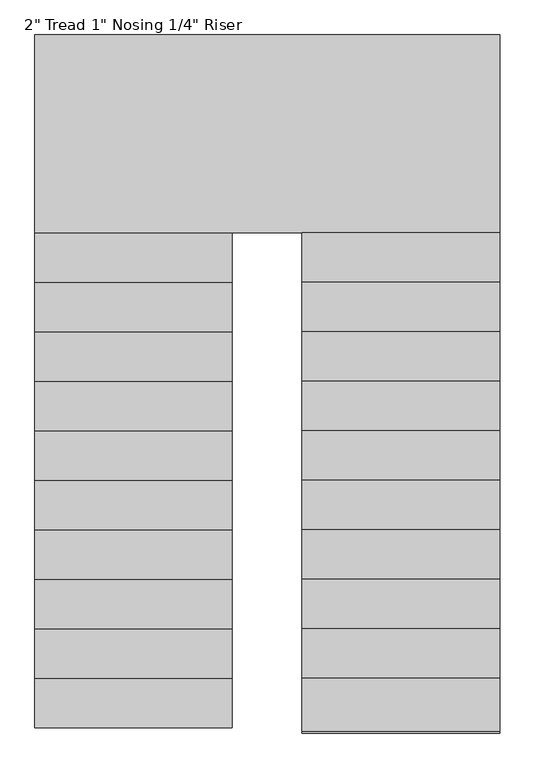
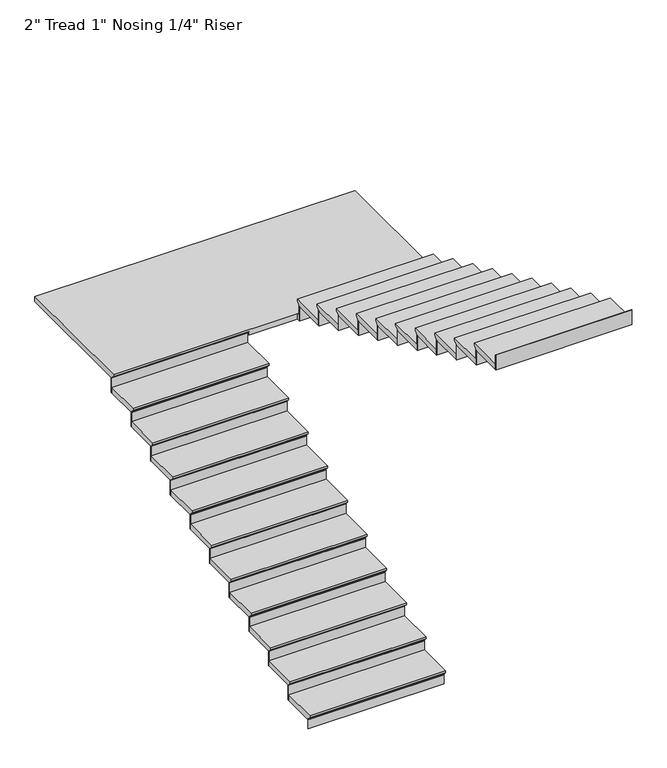
"""IFC4 building model written with IfcOpenShell, lengths in millimetres: stair flight geometry."""

from ifc_helpers import new_model, si_unit, origin, place, context, project, spatial, faceted_brep, source, transform, mapped, element, save


def stair_flight_b17f4745(model_context):
    return source(origin(), model_context, "Body", "Brep", [
        faceted_brep([(-629.5987998, 3364.6067329, 9720.6954545), (-629.5987998, 3364.6067329, 9739.7454545), (-1845.5417538, 3364.6067329, 9739.7454545), (-1845.5417538, 3364.6067329, 9720.6954545), (-629.5987998, 3390.0067329, 9695.2954545), (-1845.5417538, 3390.0067329, 9695.2954545), (-629.5987998, 3694.8067329, 9739.7454545), (-1845.5417538, 3694.8067329, 9739.7454545), (-1845.5417538, 3390.0067329, 9688.9454545), (-1845.5417538, 3694.8067329, 9688.9454545), (-629.5987998, 3694.8067329, 9688.9454545), (-629.5987998, 3390.0067329, 9688.9454545)], [[[0, 1, 2, 3]], [[4, 0, 3, 5]], [[2, 1, 6, 7]], [[8, 9, 10, 11]], [[2, 7, 9, 8, 5, 3]], [[8, 11, 4, 5]], [[6, 1, 0, 4, 11, 10]], [[7, 6, 10, 9]]]),
        faceted_brep([(-629.5987998, 3390.0067329, 9688.9454545), (-629.5987998, 3390.0067329, 9601.2), (-629.5987998, 3396.3567329, 9601.2), (-629.5987998, 3396.3567329, 9688.9454545), (-1845.5417538, 3390.0067329, 9688.9454545), (-1845.5417538, 3396.3567329, 9688.9454545), (-1845.5417538, 3396.3567329, 9601.2), (-1845.5417538, 3390.0067329, 9601.2)], [[[0, 1, 2, 3]], [[4, 5, 6, 7]], [[1, 0, 4, 7]], [[2, 1, 7, 6]], [[3, 2, 6, 5]], [[0, 3, 5, 4]]]),
        faceted_brep([(-629.5987998, 3694.8067329, 9827.4909091), (-629.5987998, 3694.8067329, 9688.9454545), (-629.5987998, 3701.1567329, 9688.9454545), (-629.5987998, 3701.1567329, 9827.4909091), (-1845.5417538, 3694.8067329, 9827.4909091), (-1845.5417538, 3701.1567329, 9827.4909091), (-1845.5417538, 3701.1567329, 9688.9454545), (-1845.5417538, 3694.8067329, 9688.9454545)], [[[0, 1, 2, 3]], [[4, 5, 6, 7]], [[1, 0, 4, 7]], [[2, 1, 7, 6]], [[3, 2, 6, 5]], [[0, 3, 5, 4]]]),
        faceted_brep([(-1845.5417538, 3669.4067329, 9878.2909091), (-629.5987998, 3669.4067329, 9878.2909091), (-629.5987998, 3999.6067329, 9878.2909091), (-1845.5417538, 3999.6067329, 9878.2909091), (-1845.5417538, 3694.8067329, 9827.4909091), (-1845.5417538, 3999.6067329, 9827.4909091), (-629.5987998, 3999.6067329, 9827.4909091), (-629.5987998, 3694.8067329, 9827.4909091), (-1845.5417538, 3694.8067329, 9833.8409091), (-1845.5417538, 3669.4067329, 9859.2409091), (-629.5987998, 3694.8067329, 9833.8409091), (-629.5987998, 3669.4067329, 9859.2409091)], [[[0, 1, 2, 3]], [[4, 5, 6, 7]], [[0, 3, 5, 4, 8, 9]], [[4, 7, 10, 8]], [[2, 1, 11, 10, 7, 6]], [[3, 2, 6, 5]], [[11, 1, 0, 9]], [[10, 11, 9, 8]]]),
        faceted_brep([(-629.5987998, 3999.6067329, 9966.0363636), (-629.5987998, 3999.6067329, 9827.4909091), (-629.5987998, 4005.9567329, 9827.4909091), (-629.5987998, 4005.9567329, 9966.0363636), (-1845.5417538, 3999.6067329, 9966.0363636), (-1845.5417538, 4005.9567329, 9966.0363636), (-1845.5417538, 4005.9567329, 9827.4909091), (-1845.5417538, 3999.6067329, 9827.4909091)], [[[0, 1, 2, 3]], [[4, 5, 6, 7]], [[1, 0, 4, 7]], [[2, 1, 7, 6]], [[3, 2, 6, 5]], [[0, 3, 5, 4]]]),
        faceted_brep([(-1845.5417538, 3974.2067329, 10016.8363636), (-629.5987998, 3974.2067329, 10016.8363636), (-629.5987998, 4304.4067329, 10016.8363636), (-1845.5417538, 4304.4067329, 10016.8363636), (-1845.5417538, 3999.6067329, 9966.0363636), (-1845.5417538, 4304.4067329, 9966.0363636), (-629.5987998, 4304.4067329, 9966.0363636), (-629.5987998, 3999.6067329, 9966.0363636), (-1845.5417538, 3999.6067329, 9972.3863636), (-1845.5417538, 3974.2067329, 9997.7863636), (-629.5987998, 3999.6067329, 9972.3863636), (-629.5987998, 3974.2067329, 9997.7863636)], [[[0, 1, 2, 3]], [[4, 5, 6, 7]], [[0, 3, 5, 4, 8, 9]], [[4, 7, 10, 8]], [[2, 1, 11, 10, 7, 6]], [[3, 2, 6, 5]], [[11, 1, 0, 9]], [[10, 11, 9, 8]]]),
        faceted_brep([(-629.5987998, 4304.4067329, 10104.5818182), (-629.5987998, 4304.4067329, 9966.0363636), (-629.5987998, 4310.7567329, 9966.0363636), (-629.5987998, 4310.7567329, 10104.5818182), (-1845.5417538, 4304.4067329, 10104.5818182), (-1845.5417538, 4310.7567329, 10104.5818182), (-1845.5417538, 4310.7567329, 9966.0363636), (-1845.5417538, 4304.4067329, 9966.0363636)], [[[0, 1, 2, 3]], [[4, 5, 6, 7]], [[1, 0, 4, 7]], [[2, 1, 7, 6]], [[3, 2, 6, 5]], [[0, 3, 5, 4]]]),
        faceted_brep([(-1845.5417538, 4279.0067329, 10155.3818182), (-629.5987998, 4279.0067329, 10155.3818182), (-629.5987998, 4609.2067329, 10155.3818182), (-1845.5417538, 4609.2067329, 10155.3818182), (-1845.5417538, 4304.4067329, 10104.5818182), (-1845.5417538, 4609.2067329, 10104.5818182), (-629.5987998, 4609.2067329, 10104.5818182), (-629.5987998, 4304.4067329, 10104.5818182), (-1845.5417538, 4304.4067329, 10110.9318182), (-1845.5417538, 4279.0067329, 10136.3318182), (-629.5987998, 4304.4067329, 10110.9318182), (-629.5987998, 4279.0067329, 10136.3318182)], [[[0, 1, 2, 3]], [[4, 5, 6, 7]], [[0, 3, 5, 4, 8, 9]], [[4, 7, 10, 8]], [[2, 1, 11, 10, 7, 6]], [[3, 2, 6, 5]], [[11, 1, 0, 9]], [[10, 11, 9, 8]]]),
        faceted_brep([(-629.5987998, 4609.2067329, 10243.1272727), (-629.5987998, 4609.2067329, 10104.5818182), (-629.5987998, 4615.5567329, 10104.5818182), (-629.5987998, 4615.5567329, 10243.1272727), (-1845.5417538, 4609.2067329, 10243.1272727), (-1845.5417538, 4615.5567329, 10243.1272727), (-1845.5417538, 4615.5567329, 10104.5818182), (-1845.5417538, 4609.2067329, 10104.5818182)], [[[0, 1, 2, 3]], [[4, 5, 6, 7]], [[1, 0, 4, 7]], [[2, 1, 7, 6]], [[3, 2, 6, 5]], [[0, 3, 5, 4]]]),
        faceted_brep([(-1845.5417538, 4583.8067329, 10293.9272727), (-629.5987998, 4583.8067329, 10293.9272727), (-629.5987998, 4914.0067329, 10293.9272727), (-1845.5417538, 4914.0067329, 10293.9272727), (-1845.5417538, 4609.2067329, 10243.1272727), (-1845.5417538, 4914.0067329, 10243.1272727), (-629.5987998, 4914.0067329, 10243.1272727), (-629.5987998, 4609.2067329, 10243.1272727), (-1845.5417538, 4609.2067329, 10249.4772727), (-1845.5417538, 4583.8067329, 10274.8772727), (-629.5987998, 4609.2067329, 10249.4772727), (-629.5987998, 4583.8067329, 10274.8772727)], [[[0, 1, 2, 3]], [[4, 5, 6, 7]], [[0, 3, 5, 4, 8, 9]], [[4, 7, 10, 8]], [[2, 1, 11, 10, 7, 6]], [[3, 2, 6, 5]], [[11, 1, 0, 9]], [[10, 11, 9, 8]]]),
        faceted_brep([(-629.5987998, 4914.0067329, 10381.6727273), (-629.5987998, 4914.0067329, 10243.1272727), (-629.5987998, 4920.3567329, 10243.1272727), (-629.5987998, 4920.3567329, 10381.6727273), (-1845.5417538, 4914.0067329, 10381.6727273), (-1845.5417538, 4920.3567329, 10381.6727273), (-1845.5417538, 4920.3567329, 10243.1272727), (-1845.5417538, 4914.0067329, 10243.1272727)], [[[0, 1, 2, 3]], [[4, 5, 6, 7]], [[1, 0, 4, 7]], [[2, 1, 7, 6]], [[3, 2, 6, 5]], [[0, 3, 5, 4]]]),
        faceted_brep([(-1845.5417538, 4888.6067329, 10432.4727273), (-629.5987998, 4888.6067329, 10432.4727273), (-629.5987998, 5218.8067329, 10432.4727273), (-1845.5417538, 5218.8067329, 10432.4727273), (-1845.5417538, 4914.0067329, 10381.6727273), (-1845.5417538, 5218.8067329, 10381.6727273), (-629.5987998, 5218.8067329, 10381.6727273), (-629.5987998, 4914.0067329, 10381.6727273), (-1845.5417538, 4914.0067329, 10388.0227273), (-1845.5417538, 4888.6067329, 10413.4227273), (-629.5987998, 4914.0067329, 10388.0227273), (-629.5987998, 4888.6067329, 10413.4227273)], [[[0, 1, 2, 3]], [[4, 5, 6, 7]], [[0, 3, 5, 4, 8, 9]], [[4, 7, 10, 8]], [[2, 1, 11, 10, 7, 6]], [[3, 2, 6, 5]], [[11, 1, 0, 9]], [[10, 11, 9, 8]]]),
        faceted_brep([(-629.5987998, 5218.8067329, 10520.2181818), (-629.5987998, 5218.8067329, 10381.6727273), (-629.5987998, 5225.1567329, 10381.6727273), (-629.5987998, 5225.1567329, 10520.2181818), (-1845.5417538, 5218.8067329, 10520.2181818), (-1845.5417538, 5225.1567329, 10520.2181818), (-1845.5417538, 5225.1567329, 10381.6727273), (-1845.5417538, 5218.8067329, 10381.6727273)], [[[0, 1, 2, 3]], [[4, 5, 6, 7]], [[1, 0, 4, 7]], [[2, 1, 7, 6]], [[3, 2, 6, 5]], [[0, 3, 5, 4]]]),
        faceted_brep([(-1845.5417538, 5193.4067329, 10571.0181818), (-629.5987998, 5193.4067329, 10571.0181818), (-629.5987998, 5523.6067329, 10571.0181818), (-1845.5417538, 5523.6067329, 10571.0181818), (-1845.5417538, 5218.8067329, 10520.2181818), (-1845.5417538, 5523.6067329, 10520.2181818), (-629.5987998, 5523.6067329, 10520.2181818), (-629.5987998, 5218.8067329, 10520.2181818), (-1845.5417538, 5218.8067329, 10526.5681818), (-1845.5417538, 5193.4067329, 10551.9681818), (-629.5987998, 5218.8067329, 10526.5681818), (-629.5987998, 5193.4067329, 10551.9681818)], [[[0, 1, 2, 3]], [[4, 5, 6, 7]], [[0, 3, 5, 4, 8, 9]], [[4, 7, 10, 8]], [[2, 1, 11, 10, 7, 6]], [[3, 2, 6, 5]], [[11, 1, 0, 9]], [[10, 11, 9, 8]]]),
        faceted_brep([(-629.5987998, 5523.6067329, 10658.7636364), (-629.5987998, 5523.6067329, 10520.2181818), (-629.5987998, 5529.9567329, 10520.2181818), (-629.5987998, 5529.9567329, 10658.7636364), (-1845.5417538, 5523.6067329, 10658.7636364), (-1845.5417538, 5529.9567329, 10658.7636364), (-1845.5417538, 5529.9567329, 10520.2181818), (-1845.5417538, 5523.6067329, 10520.2181818)], [[[0, 1, 2, 3]], [[4, 5, 6, 7]], [[1, 0, 4, 7]], [[2, 1, 7, 6]], [[3, 2, 6, 5]], [[0, 3, 5, 4]]]),
        faceted_brep([(-1845.5417538, 5498.2067329, 10709.5636364), (-629.5987998, 5498.2067329, 10709.5636364), (-629.5987998, 5828.4067329, 10709.5636364), (-1845.5417538, 5828.4067329, 10709.5636364), (-1845.5417538, 5523.6067329, 10658.7636364), (-1845.5417538, 5828.4067329, 10658.7636364), (-629.5987998, 5828.4067329, 10658.7636364), (-629.5987998, 5523.6067329, 10658.7636364), (-1845.5417538, 5523.6067329, 10665.1136364), (-1845.5417538, 5498.2067329, 10690.5136364), (-629.5987998, 5523.6067329, 10665.1136364), (-629.5987998, 5498.2067329, 10690.5136364)], [[[0, 1, 2, 3]], [[4, 5, 6, 7]], [[0, 3, 5, 4, 8, 9]], [[4, 7, 10, 8]], [[2, 1, 11, 10, 7, 6]], [[3, 2, 6, 5]], [[11, 1, 0, 9]], [[10, 11, 9, 8]]]),
        faceted_brep([(-629.5987998, 5828.4067329, 10797.3090909), (-629.5987998, 5828.4067329, 10658.7636364), (-629.5987998, 5834.7567329, 10658.7636364), (-629.5987998, 5834.7567329, 10797.3090909), (-1845.5417538, 5828.4067329, 10797.3090909), (-1845.5417538, 5834.7567329, 10797.3090909), (-1845.5417538, 5834.7567329, 10658.7636364), (-1845.5417538, 5828.4067329, 10658.7636364)], [[[0, 1, 2, 3]], [[4, 5, 6, 7]], [[1, 0, 4, 7]], [[2, 1, 7, 6]], [[3, 2, 6, 5]], [[0, 3, 5, 4]]]),
        faceted_brep([(-1845.5417538, 5803.0067329, 10848.1090909), (-629.5987998, 5803.0067329, 10848.1090909), (-629.5987998, 6133.2067329, 10848.1090909), (-1845.5417538, 6133.2067329, 10848.1090909), (-1845.5417538, 5828.4067329, 10797.3090909), (-1845.5417538, 6133.2067329, 10797.3090909), (-629.5987998, 6133.2067329, 10797.3090909), (-629.5987998, 5828.4067329, 10797.3090909), (-1845.5417538, 5828.4067329, 10803.6590909), (-1845.5417538, 5803.0067329, 10829.0590909), (-629.5987998, 5828.4067329, 10803.6590909), (-629.5987998, 5803.0067329, 10829.0590909)], [[[0, 1, 2, 3]], [[4, 5, 6, 7]], [[0, 3, 5, 4, 8, 9]], [[4, 7, 10, 8]], [[2, 1, 11, 10, 7, 6]], [[3, 2, 6, 5]], [[11, 1, 0, 9]], [[10, 11, 9, 8]]]),
        faceted_brep([(-629.5987998, 6133.2067329, 10935.8545455), (-629.5987998, 6133.2067329, 10797.3090909), (-629.5987998, 6139.5567329, 10797.3090909), (-629.5987998, 6139.5567329, 10935.8545455), (-1845.5417538, 6133.2067329, 10935.8545455), (-1845.5417538, 6139.5567329, 10935.8545455), (-1845.5417538, 6139.5567329, 10797.3090909), (-1845.5417538, 6133.2067329, 10797.3090909)], [[[0, 1, 2, 3]], [[4, 5, 6, 7]], [[1, 0, 4, 7]], [[2, 1, 7, 6]], [[3, 2, 6, 5]], [[0, 3, 5, 4]]]),
        faceted_brep([(-1845.5417538, 6107.8067329, 10986.6545455), (-629.5987998, 6107.8067329, 10986.6545455), (-629.5987998, 6438.0067329, 10986.6545455), (-1845.5417538, 6438.0067329, 10986.6545455), (-1845.5417538, 6133.2067329, 10935.8545455), (-1845.5417538, 6438.0067329, 10935.8545455), (-629.5987998, 6438.0067329, 10935.8545455), (-629.5987998, 6133.2067329, 10935.8545455), (-1845.5417538, 6133.2067329, 10942.2045455), (-1845.5417538, 6107.8067329, 10967.6045455), (-629.5987998, 6133.2067329, 10942.2045455), (-629.5987998, 6107.8067329, 10967.6045455)], [[[0, 1, 2, 3]], [[4, 5, 6, 7]], [[0, 3, 5, 4, 8, 9]], [[4, 7, 10, 8]], [[2, 1, 11, 10, 7, 6]], [[3, 2, 6, 5]], [[11, 1, 0, 9]], [[10, 11, 9, 8]]]),
        faceted_brep([(-629.5987998, 6438.0067329, 11074.4), (-629.5987998, 6438.0067329, 10935.8545455), (-629.5987998, 6444.3567329, 10935.8545455), (-629.5987998, 6444.3567329, 11074.4), (-1845.5417538, 6438.0067329, 11074.4), (-1845.5417538, 6444.3567329, 11074.4), (-1845.5417538, 6444.3567329, 10935.8545455), (-1845.5417538, 6438.0067329, 10935.8545455)], [[[0, 1, 2, 3]], [[4, 5, 6, 7]], [[1, 0, 4, 7]], [[2, 1, 7, 6]], [[3, 2, 6, 5]], [[0, 3, 5, 4]]]),
        faceted_brep([(1021.4012085, 6387.2067329, 11125.2), (1021.4012085, 7631.8067329, 11125.2), (-1845.5417538, 7631.8067329, 11125.2), (-1845.5417538, 6412.6067329, 11125.2), (-197.7987915, 6412.6067329, 11125.2), (-197.7987915, 6387.2067329, 11125.2), (1021.4012085, 7631.8067329, 11074.4), (1021.4012085, 6387.2067329, 11074.4), (-197.7987915, 6387.2067329, 11074.4), (-197.7987915, 6412.6067329, 11074.4), (-629.5987998, 6412.6067329, 11074.4), (-629.5987998, 6438.0067329, 11074.4), (-1845.5417538, 6438.0067329, 11074.4), (-1845.5417538, 7631.8067329, 11074.4), (-629.5987998, 6438.0067329, 11080.75), (-1845.5417538, 6438.0067329, 11080.75), (-1845.5417538, 6412.6067329, 11106.15), (-629.5987998, 6412.6067329, 11106.15)], [[[0, 1, 2, 3, 4, 5]], [[6, 7, 8, 9, 10, 11, 12, 13]], [[1, 0, 7, 6]], [[2, 1, 6, 13]], [[12, 11, 14, 15]], [[4, 3, 16, 17, 10, 9]], [[5, 4, 9, 8]], [[0, 5, 8, 7]], [[16, 15, 14, 17]], [[3, 2, 13, 12, 15, 16]], [[11, 10, 17, 14]]]),
        faceted_brep([(-197.7987915, 6387.2067329, 11212.9454545), (-197.7987915, 6387.2067329, 11074.4), (-197.7987915, 6380.8567329, 11074.4), (-197.7987915, 6380.8567329, 11212.9454545), (1021.4012085, 6387.2067329, 11212.9454545), (1021.4012085, 6380.8567329, 11212.9454545), (1021.4012085, 6380.8567329, 11074.4), (1021.4012085, 6387.2067329, 11074.4)], [[[0, 1, 2, 3]], [[4, 5, 6, 7]], [[1, 0, 4, 7]], [[2, 1, 7, 6]], [[3, 2, 6, 5]], [[0, 3, 5, 4]]]),
        faceted_brep([(1021.4012085, 6412.6067329, 11263.7454545), (-197.7987915, 6412.6067329, 11263.7454545), (-197.7987915, 6082.4067329, 11263.7454545), (1021.4012085, 6082.4067329, 11263.7454545), (1021.4012085, 6387.2067329, 11212.9454545), (1021.4012085, 6082.4067329, 11212.9454545), (-197.7987915, 6082.4067329, 11212.9454545), (-197.7987915, 6387.2067329, 11212.9454545), (1021.4012085, 6387.2067329, 11219.2954545), (1021.4012085, 6412.6067329, 11244.6954545), (-197.7987915, 6387.2067329, 11219.2954545), (-197.7987915, 6412.6067329, 11244.6954545)], [[[0, 1, 2, 3]], [[4, 5, 6, 7]], [[0, 3, 5, 4, 8, 9]], [[4, 7, 10, 8]], [[2, 1, 11, 10, 7, 6]], [[3, 2, 6, 5]], [[11, 1, 0, 9]], [[10, 11, 9, 8]]]),
        faceted_brep([(-197.7987915, 6082.4067329, 11351.4909091), (-197.7987915, 6082.4067329, 11212.9454545), (-197.7987915, 6076.0567329, 11212.9454545), (-197.7987915, 6076.0567329, 11351.4909091), (1021.4012085, 6082.4067329, 11351.4909091), (1021.4012085, 6076.0567329, 11351.4909091), (1021.4012085, 6076.0567329, 11212.9454545), (1021.4012085, 6082.4067329, 11212.9454545)], [[[0, 1, 2, 3]], [[4, 5, 6, 7]], [[1, 0, 4, 7]], [[2, 1, 7, 6]], [[3, 2, 6, 5]], [[0, 3, 5, 4]]]),
        faceted_brep([(1021.4012085, 6107.8067329, 11402.2909091), (-197.7987915, 6107.8067329, 11402.2909091), (-197.7987915, 5777.6067329, 11402.2909091), (1021.4012085, 5777.6067329, 11402.2909091), (1021.4012085, 6082.4067329, 11351.4909091), (1021.4012085, 5777.6067329, 11351.4909091), (-197.7987915, 5777.6067329, 11351.4909091), (-197.7987915, 6082.4067329, 11351.4909091), (1021.4012085, 6082.4067329, 11357.8409091), (1021.4012085, 6107.8067329, 11383.2409091), (-197.7987915, 6082.4067329, 11357.8409091), (-197.7987915, 6107.8067329, 11383.2409091)], [[[0, 1, 2, 3]], [[4, 5, 6, 7]], [[0, 3, 5, 4, 8, 9]], [[4, 7, 10, 8]], [[2, 1, 11, 10, 7, 6]], [[3, 2, 6, 5]], [[11, 1, 0, 9]], [[10, 11, 9, 8]]]),
        faceted_brep([(-197.7987915, 5777.6067329, 11490.0363636), (-197.7987915, 5777.6067329, 11351.4909091), (-197.7987915, 5771.2567329, 11351.4909091), (-197.7987915, 5771.2567329, 11490.0363636), (1021.4012085, 5777.6067329, 11490.0363636), (1021.4012085, 5771.2567329, 11490.0363636), (1021.4012085, 5771.2567329, 11351.4909091), (1021.4012085, 5777.6067329, 11351.4909091)], [[[0, 1, 2, 3]], [[4, 5, 6, 7]], [[1, 0, 4, 7]], [[2, 1, 7, 6]], [[3, 2, 6, 5]], [[0, 3, 5, 4]]]),
        faceted_brep([(1021.4012085, 5803.0067329, 11540.8363636), (-197.7987915, 5803.0067329, 11540.8363636), (-197.7987915, 5472.8067329, 11540.8363636), (1021.4012085, 5472.8067329, 11540.8363636), (1021.4012085, 5777.6067329, 11490.0363636), (1021.4012085, 5472.8067329, 11490.0363636), (-197.7987915, 5472.8067329, 11490.0363636), (-197.7987915, 5777.6067329, 11490.0363636), (1021.4012085, 5777.6067329, 11496.3863636), (1021.4012085, 5803.0067329, 11521.7863636), (-197.7987915, 5777.6067329, 11496.3863636), (-197.7987915, 5803.0067329, 11521.7863636)], [[[0, 1, 2, 3]], [[4, 5, 6, 7]], [[0, 3, 5, 4, 8, 9]], [[4, 7, 10, 8]], [[2, 1, 11, 10, 7, 6]], [[3, 2, 6, 5]], [[11, 1, 0, 9]], [[10, 11, 9, 8]]]),
        faceted_brep([(-197.7987915, 5472.8067329, 11628.5818182), (-197.7987915, 5472.8067329, 11490.0363636), (-197.7987915, 5466.4567329, 11490.0363636), (-197.7987915, 5466.4567329, 11628.5818182), (1021.4012085, 5472.8067329, 11628.5818182), (1021.4012085, 5466.4567329, 11628.5818182), (1021.4012085, 5466.4567329, 11490.0363636), (1021.4012085, 5472.8067329, 11490.0363636)], [[[0, 1, 2, 3]], [[4, 5, 6, 7]], [[1, 0, 4, 7]], [[2, 1, 7, 6]], [[3, 2, 6, 5]], [[0, 3, 5, 4]]]),
        faceted_brep([(1021.4012085, 5498.2067329, 11679.3818182), (-197.7987915, 5498.2067329, 11679.3818182), (-197.7987915, 5168.0067329, 11679.3818182), (1021.4012085, 5168.0067329, 11679.3818182), (1021.4012085, 5472.8067329, 11628.5818182), (1021.4012085, 5168.0067329, 11628.5818182), (-197.7987915, 5168.0067329, 11628.5818182), (-197.7987915, 5472.8067329, 11628.5818182), (1021.4012085, 5472.8067329, 11634.9318182), (1021.4012085, 5498.2067329, 11660.3318182), (-197.7987915, 5472.8067329, 11634.9318182), (-197.7987915, 5498.2067329, 11660.3318182)], [[[0, 1, 2, 3]], [[4, 5, 6, 7]], [[0, 3, 5, 4, 8, 9]], [[4, 7, 10, 8]], [[2, 1, 11, 10, 7, 6]], [[3, 2, 6, 5]], [[11, 1, 0, 9]], [[10, 11, 9, 8]]]),
        faceted_brep([(-197.7987915, 5168.0067329, 11767.1272727), (-197.7987915, 5168.0067329, 11628.5818182), (-197.7987915, 5161.6567329, 11628.5818182), (-197.7987915, 5161.6567329, 11767.1272727), (1021.4012085, 5168.0067329, 11767.1272727), (1021.4012085, 5161.6567329, 11767.1272727), (1021.4012085, 5161.6567329, 11628.5818182), (1021.4012085, 5168.0067329, 11628.5818182)], [[[0, 1, 2, 3]], [[4, 5, 6, 7]], [[1, 0, 4, 7]], [[2, 1, 7, 6]], [[3, 2, 6, 5]], [[0, 3, 5, 4]]]),
        faceted_brep([(1021.4012085, 5193.4067329, 11817.9272727), (-197.7987915, 5193.4067329, 11817.9272727), (-197.7987915, 4863.2067329, 11817.9272727), (1021.4012085, 4863.2067329, 11817.9272727), (1021.4012085, 5168.0067329, 11767.1272727), (1021.4012085, 4863.2067329, 11767.1272727), (-197.7987915, 4863.2067329, 11767.1272727), (-197.7987915, 5168.0067329, 11767.1272727), (1021.4012085, 5168.0067329, 11773.4772727), (1021.4012085, 5193.4067329, 11798.8772727), (-197.7987915, 5168.0067329, 11773.4772727), (-197.7987915, 5193.4067329, 11798.8772727)], [[[0, 1, 2, 3]], [[4, 5, 6, 7]], [[0, 3, 5, 4, 8, 9]], [[4, 7, 10, 8]], [[2, 1, 11, 10, 7, 6]], [[3, 2, 6, 5]], [[11, 1, 0, 9]], [[10, 11, 9, 8]]]),
        faceted_brep([(-197.7987915, 4863.2067329, 11905.6727273), (-197.7987915, 4863.2067329, 11767.1272727), (-197.7987915, 4856.8567329, 11767.1272727), (-197.7987915, 4856.8567329, 11905.6727273), (1021.4012085, 4863.2067329, 11905.6727273), (1021.4012085, 4856.8567329, 11905.6727273), (1021.4012085, 4856.8567329, 11767.1272727), (1021.4012085, 4863.2067329, 11767.1272727)], [[[0, 1, 2, 3]], [[4, 5, 6, 7]], [[1, 0, 4, 7]], [[2, 1, 7, 6]], [[3, 2, 6, 5]], [[0, 3, 5, 4]]]),
        faceted_brep([(1021.4012085, 4888.6067329, 11956.4727273), (-197.7987915, 4888.6067329, 11956.4727273), (-197.7987915, 4558.4067329, 11956.4727273), (1021.4012085, 4558.4067329, 11956.4727273), (1021.4012085, 4863.2067329, 11905.6727273), (1021.4012085, 4558.4067329, 11905.6727273), (-197.7987915, 4558.4067329, 11905.6727273), (-197.7987915, 4863.2067329, 11905.6727273), (1021.4012085, 4863.2067329, 11912.0227273), (1021.4012085, 4888.6067329, 11937.4227273), (-197.7987915, 4863.2067329, 11912.0227273), (-197.7987915, 4888.6067329, 11937.4227273)], [[[0, 1, 2, 3]], [[4, 5, 6, 7]], [[0, 3, 5, 4, 8, 9]], [[4, 7, 10, 8]], [[2, 1, 11, 10, 7, 6]], [[3, 2, 6, 5]], [[11, 1, 0, 9]], [[10, 11, 9, 8]]]),
        faceted_brep([(-197.7987915, 4558.4067329, 12044.2181818), (-197.7987915, 4558.4067329, 11905.6727273), (-197.7987915, 4552.0567329, 11905.6727273), (-197.7987915, 4552.0567329, 12044.2181818), (1021.4012085, 4558.4067329, 12044.2181818), (1021.4012085, 4552.0567329, 12044.2181818), (1021.4012085, 4552.0567329, 11905.6727273), (1021.4012085, 4558.4067329, 11905.6727273)], [[[0, 1, 2, 3]], [[4, 5, 6, 7]], [[1, 0, 4, 7]], [[2, 1, 7, 6]], [[3, 2, 6, 5]], [[0, 3, 5, 4]]]),
        faceted_brep([(1021.4012085, 4583.8067329, 12095.0181818), (-197.7987915, 4583.8067329, 12095.0181818), (-197.7987915, 4253.6067329, 12095.0181818), (1021.4012085, 4253.6067329, 12095.0181818), (1021.4012085, 4558.4067329, 12044.2181818), (1021.4012085, 4253.6067329, 12044.2181818), (-197.7987915, 4253.6067329, 12044.2181818), (-197.7987915, 4558.4067329, 12044.2181818), (1021.4012085, 4558.4067329, 12050.5681818), (1021.4012085, 4583.8067329, 12075.9681818), (-197.7987915, 4558.4067329, 12050.5681818), (-197.7987915, 4583.8067329, 12075.9681818)], [[[0, 1, 2, 3]], [[4, 5, 6, 7]], [[0, 3, 5, 4, 8, 9]], [[4, 7, 10, 8]], [[2, 1, 11, 10, 7, 6]], [[3, 2, 6, 5]], [[11, 1, 0, 9]], [[10, 11, 9, 8]]]),
        faceted_brep([(-197.7987915, 4253.6067329, 12182.7636364), (-197.7987915, 4253.6067329, 12044.2181818), (-197.7987915, 4247.2567329, 12044.2181818), (-197.7987915, 4247.2567329, 12182.7636364), (1021.4012085, 4253.6067329, 12182.7636364), (1021.4012085, 4247.2567329, 12182.7636364), (1021.4012085, 4247.2567329, 12044.2181818), (1021.4012085, 4253.6067329, 12044.2181818)], [[[0, 1, 2, 3]], [[4, 5, 6, 7]], [[1, 0, 4, 7]], [[2, 1, 7, 6]], [[3, 2, 6, 5]], [[0, 3, 5, 4]]]),
        faceted_brep([(1021.4012085, 4279.0067329, 12233.5636364), (-197.7987915, 4279.0067329, 12233.5636364), (-197.7987915, 3948.8067329, 12233.5636364), (1021.4012085, 3948.8067329, 12233.5636364), (1021.4012085, 4253.6067329, 12182.7636364), (1021.4012085, 3948.8067329, 12182.7636364), (-197.7987915, 3948.8067329, 12182.7636364), (-197.7987915, 4253.6067329, 12182.7636364), (1021.4012085, 4253.6067329, 12189.1136364), (1021.4012085, 4279.0067329, 12214.5136364), (-197.7987915, 4253.6067329, 12189.1136364), (-197.7987915, 4279.0067329, 12214.5136364)], [[[0, 1, 2, 3]], [[4, 5, 6, 7]], [[0, 3, 5, 4, 8, 9]], [[4, 7, 10, 8]], [[2, 1, 11, 10, 7, 6]], [[3, 2, 6, 5]], [[11, 1, 0, 9]], [[10, 11, 9, 8]]]),
        faceted_brep([(-197.7987915, 3948.8067329, 12321.3090909), (-197.7987915, 3948.8067329, 12182.7636364), (-197.7987915, 3942.4567329, 12182.7636364), (-197.7987915, 3942.4567329, 12321.3090909), (1021.4012085, 3948.8067329, 12321.3090909), (1021.4012085, 3942.4567329, 12321.3090909), (1021.4012085, 3942.4567329, 12182.7636364), (1021.4012085, 3948.8067329, 12182.7636364)], [[[0, 1, 2, 3]], [[4, 5, 6, 7]], [[1, 0, 4, 7]], [[2, 1, 7, 6]], [[3, 2, 6, 5]], [[0, 3, 5, 4]]]),
        faceted_brep([(1021.4012085, 3974.2067329, 12372.1090909), (-197.7987915, 3974.2067329, 12372.1090909), (-197.7987915, 3644.0067329, 12372.1090909), (1021.4012085, 3644.0067329, 12372.1090909), (1021.4012085, 3948.8067329, 12321.3090909), (1021.4012085, 3644.0067329, 12321.3090909), (-197.7987915, 3644.0067329, 12321.3090909), (-197.7987915, 3948.8067329, 12321.3090909), (1021.4012085, 3948.8067329, 12327.6590909), (1021.4012085, 3974.2067329, 12353.0590909), (-197.7987915, 3948.8067329, 12327.6590909), (-197.7987915, 3974.2067329, 12353.0590909)], [[[0, 1, 2, 3]], [[4, 5, 6, 7]], [[0, 3, 5, 4, 8, 9]], [[4, 7, 10, 8]], [[2, 1, 11, 10, 7, 6]], [[3, 2, 6, 5]], [[11, 1, 0, 9]], [[10, 11, 9, 8]]]),
        faceted_brep([(-197.7987915, 3644.0067329, 12459.8545455), (-197.7987915, 3644.0067329, 12321.3090909), (-197.7987915, 3637.6567329, 12321.3090909), (-197.7987915, 3637.6567329, 12459.8545455), (1021.4012085, 3644.0067329, 12459.8545455), (1021.4012085, 3637.6567329, 12459.8545455), (1021.4012085, 3637.6567329, 12321.3090909), (1021.4012085, 3644.0067329, 12321.3090909)], [[[0, 1, 2, 3]], [[4, 5, 6, 7]], [[1, 0, 4, 7]], [[2, 1, 7, 6]], [[3, 2, 6, 5]], [[0, 3, 5, 4]]]),
        faceted_brep([(-197.7987915, 3339.2067329, 12598.4), (-197.7987915, 3339.2067329, 12459.8545455), (-197.7987915, 3332.8567329, 12459.8545455), (-197.7987915, 3332.8567329, 12598.4), (1021.4012085, 3339.2067329, 12598.4), (1021.4012085, 3332.8567329, 12598.4), (1021.4012085, 3332.8567329, 12459.8545455), (1021.4012085, 3339.2067329, 12459.8545455)], [[[0, 1, 2, 3]], [[4, 5, 6, 7]], [[1, 0, 4, 7]], [[2, 1, 7, 6]], [[3, 2, 6, 5]], [[0, 3, 5, 4]]]),
        faceted_brep([(1021.4012085, 3669.4067329, 12510.6545455), (-197.7987915, 3669.4067329, 12510.6545455), (-197.7987915, 3339.2067329, 12510.6545455), (1021.4012085, 3339.2067329, 12510.6545455), (1021.4012085, 3644.0067329, 12459.8545455), (1021.4012085, 3339.2067329, 12459.8545455), (-197.7987915, 3339.2067329, 12459.8545455), (-197.7987915, 3644.0067329, 12459.8545455), (1021.4012085, 3644.0067329, 12466.2045455), (1021.4012085, 3669.4067329, 12491.6045455), (-197.7987915, 3644.0067329, 12466.2045455), (-197.7987915, 3669.4067329, 12491.6045455)], [[[0, 1, 2, 3]], [[4, 5, 6, 7]], [[0, 3, 5, 4, 8, 9]], [[4, 7, 10, 8]], [[2, 1, 11, 10, 7, 6]], [[3, 2, 6, 5]], [[11, 1, 0, 9]], [[10, 11, 9, 8]]]),
    ])


if __name__ == "__main__":
    model = new_model("IFC4")
    model_context = context("Model", 3, world=origin())
    ifc_project = project(units=[si_unit("LENGTHUNIT", "METRE", prefix="MILLI")], contexts=[model_context])
    site = spatial("IfcSite", under=ifc_project)
    building = spatial("IfcBuilding", under=site)
    placement = place(None, origin())
    stair_flight_shape = stair_flight_b17f4745(model_context)
    element("IfcStairFlight", 1, ObjectType="2\" Tread 1\" Nosing 1/4\" Riser", at=placement, inside=building, context=model_context, shape_type="MappedRepresentation", body=[
        mapped(stair_flight_shape, transform((0.0, 0.0, 0.0), x_axis=(1.0, 0.0, 0.0), y_axis=(0.0, 1.0, 0.0), z_axis=(0.0, 0.0, 1.0))),
    ])
    save(model, "model.ifc")
